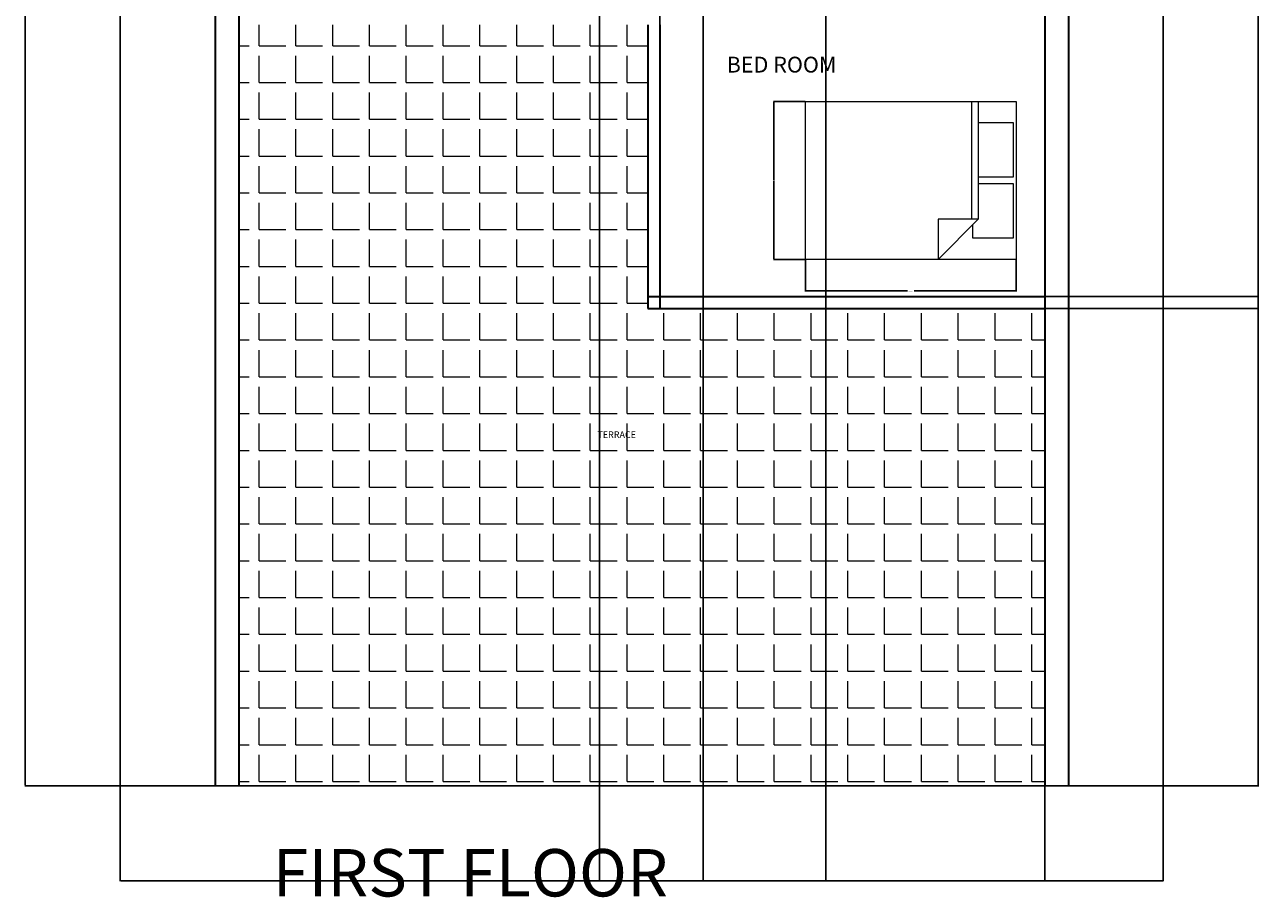
# Model space of a CAD drawing. Units: inches. Extents: x 2621 to 3621, y 1701 to 2465.
# Tile 5 of 6: x 3152 to 3621, y 1702 to 2034. Entities that reach past the tile are written whole.
import ezdxf

# ---------------------------------------------------------------- set-up
doc = ezdxf.new("R2010")
doc.units = ezdxf.units.IN
for name, color, linetype, lineweight in [('A-ANNO-DIMS', 2, 'Continuous', 18), ('A-ANNO-TEXT', 7, 'Continuous', 25), ('A-AREA-IDEN', 7, 'Continuous', 18), ('A-FLOR-PATT', 252, 'Continuous', 13), ('A-FURN', 8, 'Continuous', 18), ('A-WALL', 7, 'Continuous', 35), ('C-PROP', 8, 'Continuous', 25)]:
    doc.layers.add(name, color=color, linetype=linetype, lineweight=lineweight)
doc.styles.get("Standard").update_dxf_attribs({"font": 'arial.ttf'})
doc.dimstyles.get("Standard").update_dxf_attribs({"dimtxt": 0.18, "dimasz": 0.18, "dimexe": 0.18, "dimexo": 0.0625, "dimgap": 0.09, "dimtad": 0, "dimtih": 1, "dimtoh": 1, "dimdec": 4, "dimzin": 0, "dimdsep": 46, "dimtxsty": 'Standard', "dimcen": 0.09, "dimadec": 0, "dimazin": 0, "dimtfac": 1, "dimtdec": 4, "dimtofl": 0, "dimtmove": 0, "dimatfit": 3, "dimfxl": 1, "dimtolj": 1, "dimtzin": 0, "dimarcsym": 0})

# ---------------------------------------------------------------- blocks, each defined once
blk = doc.blocks.new('Bed - Queen')
for p, q in [((0, -80.00003), (0, 0)), ((0, 0), (59.99999, 0)), ((59.99999, 0), (59.99999, -80.00003)), ((7.99999, -1.2), (28.79998, -1.2)), ((7.99999, -14.4), (7.99999, -1.2)), ((28.79998, -1.2), (28.79998, -14.4)), ((31.19999, -1.2), (51.99999, -1.2)), ((31.19999, -14.4), (31.19999, -1.2)), ((51.99999, -1.2), (51.99999, -16.4)), ((0, -14.4), (44.8, -14.4)), ((44.8, -16.8), (0, -16.8)), ((59.99999, -29.6), (44.8, -14.4)), ((44.8, -14.4), (44.8, -29.6)), ((51.99999, -16.4), (46.79936, -16.4)), ((44.8, -29.6), (59.99999, -29.6)), ((59.99999, -80.00003), (0, -80.00003))]:
    blk.add_line(p, q)
blk = doc.blocks.new('LOT-33X57')
for p, q in [((0, 684), (396, 684)), ((0, 0), (0, 684)), ((396, 684), (396, 0)), ((396, 0), (0, 0))]:
    blk.add_line(p, q)
blk = doc.blocks.new('*D15')
at = {"layer": 'A-ANNO-DIMS', "color": 0, "lineweight": -2, "transparency": 16777216}
for p, q in [((3448.49, 1944.46), (3448.49, 1932.34)), ((3528.49, 1944.46), (3528.49, 1932.34)), ((3448.67, 1932.52), (3487.18, 1932.52)), ((3528.31, 1932.52), (3489.79, 1932.52))]:
    blk.add_line(p, q, dxfattribs=at)
at = {"layer": 'A-ANNO-DIMS', "color": 0, "transparency": 16777216}
for points in [[(3448.67, 1932.55), (3448.67, 1932.49), (3448.49, 1932.52)], [(3528.31, 1932.55), (3528.31, 1932.49), (3528.49, 1932.52)]]:
    blk.add_solid(points, dxfattribs=at)
at = {"layer": 'Defpoints', "color": 0, "transparency": 16777216}
for p in [(3448.49, 1944.52), (3528.49, 1944.52), (3528.49, 1932.52)]:
    blk.add_point(p, dxfattribs=at)
at = {"layer": 'A-ANNO-DIMS', "color": 0, "transparency": 16777216, "insert": (3488.49, 1932.52), "char_height": 0.18, "attachment_point": 5}
blk.add_mtext('\\A1;QUEEN BED 80 TYP.', dxfattribs=at)
blk = doc.blocks.new('*D16')
at = {"layer": 'A-ANNO-DIMS', "color": 0, "lineweight": -2, "transparency": 16777216}
for p, q in [((3448.43, 2004.52), (3436.31, 2004.52)), ((3436.49, 2004.34), (3436.49, 1974.7)), ((3436.49, 1944.7), (3436.49, 1974.34)), ((3448.43, 1944.52), (3436.31, 1944.52))]:
    blk.add_line(p, q, dxfattribs=at)
at = {"layer": 'A-ANNO-DIMS', "color": 0, "transparency": 16777216}
for points in [[(3436.46, 2004.34), (3436.52, 2004.34), (3436.49, 2004.52)], [(3436.46, 1944.7), (3436.52, 1944.7), (3436.49, 1944.52)]]:
    blk.add_solid(points, dxfattribs=at)
at = {"layer": 'Defpoints', "color": 0, "transparency": 16777216}
for p in [(3448.49, 2004.52), (3436.49, 1944.52), (3448.49, 1944.52)]:
    blk.add_point(p, dxfattribs=at)
at = {"layer": 'A-ANNO-DIMS', "color": 0, "transparency": 16777216, "insert": (3436.49, 1974.52), "char_height": 0.18, "attachment_point": 5}
blk.add_mtext('\\A1;60 TYP.', dxfattribs=at)
blk = doc.blocks.new('*D63')
at = {"layer": 'A-ANNO-DIMS', "color": 0, "lineweight": -2, "transparency": 16777216}
for p, q in [((3188.33, 1744.56), (3188.33, 1708.36)), ((3584.33, 1744.56), (3584.33, 1708.36)), ((3188.51, 1708.54), (3386.05, 1708.54)), ((3584.15, 1708.54), (3386.62, 1708.54))]:
    blk.add_line(p, q, dxfattribs=at)
at = {"layer": 'A-ANNO-DIMS', "color": 0, "transparency": 16777216}
for points in [[(3188.51, 1708.57), (3188.51, 1708.51), (3188.33, 1708.54)], [(3584.15, 1708.57), (3584.15, 1708.51), (3584.33, 1708.54)]]:
    blk.add_solid(points, dxfattribs=at)
at = {"layer": 'Defpoints', "color": 0, "transparency": 16777216}
for p in [(3188.33, 1744.63), (3584.33, 1744.63), (3584.33, 1708.54)]:
    blk.add_point(p, dxfattribs=at)
at = {"layer": 'A-ANNO-DIMS', "color": 0, "transparency": 16777216, "insert": (3386.33, 1708.54), "char_height": 0.18, "attachment_point": 5}
blk.add_mtext('\\A1;396', dxfattribs=at)
blk = doc.blocks.new('*D64')
at = {"layer": 'A-ANNO-DIMS', "color": 0, "lineweight": -2, "transparency": 16777216}
for p, q in [((3188.27, 2428.63), (3152.07, 2428.63)), ((3152.25, 2428.45), (3152.25, 2086.81)), ((3152.25, 1744.81), (3152.25, 2086.44)), ((3188.27, 1744.63), (3152.07, 1744.63))]:
    blk.add_line(p, q, dxfattribs=at)
at = {"layer": 'A-ANNO-DIMS', "color": 0, "transparency": 16777216}
for points in [[(3152.22, 2428.45), (3152.28, 2428.45), (3152.25, 2428.63)], [(3152.22, 1744.81), (3152.28, 1744.81), (3152.25, 1744.63)]]:
    blk.add_solid(points, dxfattribs=at)
at = {"layer": 'Defpoints', "color": 0, "transparency": 16777216}
for p in [(3152.25, 2428.63), (3188.33, 2428.63), (3188.33, 1744.63)]:
    blk.add_point(p, dxfattribs=at)
at = {"layer": 'A-ANNO-DIMS', "color": 0, "transparency": 16777216, "insert": (3152.25, 2086.63), "char_height": 0.18, "attachment_point": 5}
blk.add_mtext('\\A1;684', dxfattribs=at)
blk = doc.blocks.new('*D66')
at = {"layer": 'A-ANNO-DIMS', "color": 0, "lineweight": -2, "transparency": 16777216}
for p, q in [((3548.4, 2392.63), (3620.6, 2392.63)), ((3620.42, 2392.45), (3620.42, 2068.81)), ((3620.42, 1744.81), (3620.42, 2068.44)), ((3548.4, 1744.63), (3620.6, 1744.63))]:
    blk.add_line(p, q, dxfattribs=at)
at = {"layer": 'A-ANNO-DIMS', "color": 0, "transparency": 16777216}
for points in [[(3620.39, 2392.45), (3620.45, 2392.45), (3620.42, 2392.63)], [(3620.39, 1744.81), (3620.45, 1744.81), (3620.42, 1744.63)]]:
    blk.add_solid(points, dxfattribs=at)
at = {"layer": 'Defpoints', "color": 0, "transparency": 16777216}
for p in [(3548.33, 2392.63), (3620.42, 2392.63), (3548.33, 1744.63)]:
    blk.add_point(p, dxfattribs=at)
at = {"layer": 'A-ANNO-DIMS', "color": 0, "transparency": 16777216, "insert": (3620.42, 2068.63), "char_height": 0.18, "attachment_point": 5}
blk.add_mtext('\\A1;648', dxfattribs=at)
blk = doc.blocks.new('*D68')
at = {"layer": 'A-ANNO-DIMS', "color": 0, "lineweight": -2, "transparency": 16777216}
for p, q in [((3370.34, 2383.56), (3370.34, 1708.36)), ((3409.59, 2383.56), (3409.59, 1708.36)), ((3370.52, 1708.54), (3389.57, 1708.54)), ((3409.41, 1708.54), (3390.36, 1708.54))]:
    blk.add_line(p, q, dxfattribs=at)
at = {"layer": 'A-ANNO-DIMS', "color": 0, "transparency": 16777216}
for points in [[(3370.52, 1708.57), (3370.52, 1708.51), (3370.34, 1708.54)], [(3409.41, 1708.57), (3409.41, 1708.51), (3409.59, 1708.54)]]:
    blk.add_solid(points, dxfattribs=at)
at = {"layer": 'Defpoints', "color": 0, "transparency": 16777216}
for p in [(3370.34, 2383.63), (3409.59, 2383.63), (3409.59, 1708.54)]:
    blk.add_point(p, dxfattribs=at)
at = {"layer": 'A-ANNO-DIMS', "color": 0, "transparency": 16777216, "insert": (3389.97, 1708.54), "char_height": 0.18, "attachment_point": 5}
blk.add_mtext('\\A1;39.25', dxfattribs=at)
blk = doc.blocks.new('*D76')
at = {"layer": 'A-ANNO-DIMS', "color": 0, "lineweight": -2, "transparency": 16777216}
for p, q in [((3456.23, 2062.74), (3456.23, 1708.36)), ((3539.33, 2062.74), (3539.33, 1708.36)), ((3456.41, 1708.54), (3497.47, 1708.54)), ((3539.15, 1708.54), (3498.09, 1708.54))]:
    blk.add_line(p, q, dxfattribs=at)
at = {"layer": 'A-ANNO-DIMS', "color": 0, "transparency": 16777216}
for points in [[(3456.41, 1708.57), (3456.41, 1708.51), (3456.23, 1708.54)], [(3539.15, 1708.57), (3539.15, 1708.51), (3539.33, 1708.54)]]:
    blk.add_solid(points, dxfattribs=at)
at = {"layer": 'Defpoints', "color": 0, "transparency": 16777216}
for p in [(3456.23, 2062.8), (3539.33, 2062.8), (3539.33, 1708.54)]:
    blk.add_point(p, dxfattribs=at)
at = {"layer": 'A-ANNO-DIMS', "color": 0, "transparency": 16777216, "insert": (3497.78, 1708.54), "char_height": 0.18, "attachment_point": 5}
blk.add_mtext('\\A1;83.1', dxfattribs=at)
blk = doc.blocks.new('*D78')
at = {"layer": 'A-ANNO-DIMS', "color": 0, "lineweight": -2, "transparency": 16777216}
for p, q in [((3393.19, 1925.94), (3393.19, 2464.89)), ((3393.37, 2464.71), (3465.81, 2464.71)), ((3539.15, 2464.71), (3466.72, 2464.71)), ((3539.33, 1930.44), (3539.33, 2464.89))]:
    blk.add_line(p, q, dxfattribs=at)
at = {"layer": 'A-ANNO-DIMS', "color": 0, "transparency": 16777216}
for points in [[(3393.37, 2464.74), (3393.37, 2464.68), (3393.19, 2464.71)], [(3539.15, 2464.74), (3539.15, 2464.68), (3539.33, 2464.71)]]:
    blk.add_solid(points, dxfattribs=at)
at = {"layer": 'Defpoints', "color": 0, "transparency": 16777216}
for p in [(3539.33, 2464.71), (3539.33, 1930.38), (3393.19, 1925.88)]:
    blk.add_point(p, dxfattribs=at)
at = {"layer": 'A-ANNO-DIMS', "color": 0, "transparency": 16777216, "insert": (3466.26, 2464.71), "char_height": 0.18, "attachment_point": 5}
blk.add_mtext('\\A1;146.14', dxfattribs=at)
blk = doc.blocks.new('*D79')
at = {"layer": 'A-ANNO-DIMS', "color": 0, "lineweight": -2, "transparency": 16777216}
for p, q in [((3539.4, 2062.8), (3620.6, 2062.8)), ((3620.42, 2062.62), (3620.42, 1996.77)), ((3620.42, 1930.56), (3620.42, 1996.41)), ((3539.4, 1930.38), (3620.6, 1930.38))]:
    blk.add_line(p, q, dxfattribs=at)
at = {"layer": 'A-ANNO-DIMS', "color": 0, "transparency": 16777216}
for points in [[(3620.39, 2062.62), (3620.45, 2062.62), (3620.42, 2062.8)], [(3620.39, 1930.56), (3620.45, 1930.56), (3620.42, 1930.38)]]:
    blk.add_solid(points, dxfattribs=at)
at = {"layer": 'Defpoints', "color": 0, "transparency": 16777216}
for p in [(3539.33, 2062.8), (3620.42, 2062.8), (3539.33, 1930.38)]:
    blk.add_point(p, dxfattribs=at)
at = {"layer": 'A-ANNO-DIMS', "color": 0, "transparency": 16777216, "insert": (3620.42, 1996.59), "char_height": 0.18, "attachment_point": 5}
blk.add_mtext('\\A1;132.42', dxfattribs=at)
blk = doc.blocks.new('*D80')
at = {"layer": 'A-ANNO-DIMS', "color": 0, "lineweight": -2, "transparency": 16777216}
for p, q in [((3539.4, 1925.88), (3620.6, 1925.88)), ((3620.42, 1925.7), (3620.42, 1835.44)), ((3620.42, 1744.81), (3620.42, 1835.07)), ((3539.4, 1744.63), (3620.6, 1744.63))]:
    blk.add_line(p, q, dxfattribs=at)
at = {"layer": 'A-ANNO-DIMS', "color": 0, "transparency": 16777216}
for points in [[(3620.39, 1925.7), (3620.45, 1925.7), (3620.42, 1925.88)], [(3620.39, 1744.81), (3620.45, 1744.81), (3620.42, 1744.63)]]:
    blk.add_solid(points, dxfattribs=at)
at = {"layer": 'Defpoints', "color": 0, "transparency": 16777216}
for p in [(3539.33, 1925.88), (3620.42, 1925.88), (3539.33, 1744.63)]:
    blk.add_point(p, dxfattribs=at)
at = {"layer": 'A-ANNO-DIMS', "color": 0, "transparency": 16777216, "insert": (3620.42, 1835.25), "char_height": 0.18, "attachment_point": 5}
blk.add_mtext('\\A1;181.26', dxfattribs=at)

msp = doc.modelspace()

# ---------------------------------------------------------------- hatches: boundary and pattern name
at = {"layer": 'A-FLOR-PATT'}
h = msp.add_hatch(dxfattribs=at)
h.set_pattern_fill('ANGLE', color=256, scale=2)
h.set_pattern_definition([(0, (0, 0), (0, 13.97), [10.16, -3.81]), (90, (0, 0), (-13.97, 9e-16), [10.16, -3.81])])
h.paths.add_polyline_path([(3233.335, 2383.626), (3233.335, 2215.626), (3366.0915, 2215.626), (3366.0915, 2383.626), (3344.3345, 2383.626), (3339.8345, 2383.626)])
h.paths.add_polyline_path([(3233.335, 2033.6278), (3233.335, 1895.6231), (3233.335, 1744.626), (3539.335, 1744.626), (3539.335, 1780.626), (3539.335, 1789.626), (3539.335, 1859.7646), (3539.335, 1862.3069), (3539.335, 1925.8819), (3388.6903, 1925.8819), (3388.6903, 2033.6278)])

# ---------------------------------------------------------------- linework, layer by layer
at = {"layer": 'A-WALL'}
for p, q in [((3224.335, 2428.626), (3224.335, 1891.1231)), ((3233.335, 2111.9772), (3233.335, 1895.6231)), ((3539.335, 2111.9772), (3539.335, 2015.622)), ((3548.335, 2111.9772), (3548.335, 1780.626)), ((3388.6903, 2033.6278), (3388.6903, 1925.8819)), ((3393.1903, 2033.6278), (3393.1903, 1925.8819)), ((3539.335, 2015.622), (3539.335, 2011.122)), ((3539.335, 2011.122), (3539.335, 1955.3016)), ((3539.335, 1955.3016), (3539.335, 1950.8016)), ((3539.335, 1950.8016), (3539.335, 1862.3069)), ((3388.6903, 1930.3819), (3539.335, 1930.3819)), ((3388.6903, 1925.8819), (3539.335, 1925.8819)), ((3233.335, 1895.6231), (3233.335, 1744.626)), ((3224.335, 1891.1231), (3224.335, 1744.626)), ((3539.335, 1862.3069), (3539.335, 1859.7646)), ((3539.335, 1859.7646), (3539.335, 1789.626)), ((3539.335, 1789.626), (3539.335, 1780.626)), ((3539.335, 1780.626), (3539.335, 1744.626)), ((3548.335, 1780.626), (3548.335, 1744.626))]:
    msp.add_line(p, q, dxfattribs=at)

# ---------------------------------------------------------------- block references
at = {"layer": 'A-FURN', "rotation": 270}
msp.add_blockref('Bed - Queen', (3528.4879, 2004.5213), dxfattribs=at)
at = {"layer": 'C-PROP'}
msp.add_blockref('LOT-33X57', (3188.3346, 1744.6265), dxfattribs=at)

# ---------------------------------------------------------------- texts
at = {"layer": 'A-ANNO-TEXT', "insert": (3246.1971, 1720.589), "char_height": 18, "attachment_point": 1}
msp.add_mtext_dynamic_manual_height_columns('FIRST FLOOR', width=483.442651, gutter_width=12.5, heights=[0], dxfattribs=at)
at = {"layer": 'A-AREA-IDEN', "attachment_point": 1}
for s, width, insert, char_height in [('BED ROOM', 49.051461, (3418.5714, 2021.4596), 6), ('TERRACE ', 54.244428, (3369.4942, 1879.2046), 2.5)]:
    msp.add_mtext_dynamic_manual_height_columns(s, width=width, gutter_width=12.5, heights=[0], dxfattribs=dict(at, insert=insert, char_height=char_height))

# ---------------------------------------------------------------- dimensions: what is measured, and where the dimension line sits
at = {"layer": 'A-ANNO-DIMS'}
for base, p1, p2, override, picture, middle in [((3539.335, 2464.708), (3393.1903, 1925.8819), (3539.335, 1930.3819), {"dimdec": 2, "dimlfac": 1, "dimrnd": 0, "dimzin": 0, "dimdsep": 46, "dimlunit": 2}, '*D78', (3466.2626, 2464.708)), ((3409.5915, 1708.544), (3370.3415, 2383.626), (3409.5915, 2383.626), {"dimdec": 2, "dimlfac": 1, "dimrnd": 0, "dimzin": 0, "dimdsep": 46, "dimlunit": 2}, '*D68', (3389.9665, 1708.544)), ((3539.335, 1708.544), (3456.2276, 2062.7992), (3539.335, 2062.7992), {"dimdec": 1, "dimlfac": 1, "dimrnd": 0, "dimzin": 0, "dimdsep": 46, "dimlunit": 2}, '*D76', (3497.7813, 1708.544)), ((3584.335, 1708.544), (3188.335, 1744.626), (3584.335, 1744.626), {"dimdec": 0, "dimlfac": 1, "dimrnd": 0, "dimzin": 0, "dimdsep": 46, "dimlunit": 2}, '*D63', (3386.335, 1708.544))]:
    dim = msp.add_linear_dim(base=base, p1=p1, p2=p2, dimstyle='Standard', override=override, dxfattribs=at)
    dim.commit()
    dim.dimension.update_dxf_attribs({"geometry": picture, "text_midpoint": middle})
for base, p1, p2, override, picture, middle in [((3152.253, 2428.626), (3188.335, 1744.626), (3188.335, 2428.626), {"dimdec": 0, "dimlfac": 1, "dimrnd": 0, "dimzin": 0, "dimdsep": 46, "dimlunit": 2}, '*D64', (3152.253, 2086.626)), ((3620.417, 2392.626), (3548.335, 1744.626), (3548.335, 2392.626), {"dimdec": 0, "dimlfac": 1, "dimrnd": 0, "dimzin": 0, "dimdsep": 46, "dimlunit": 2}, '*D66', (3620.417, 2068.626)), ((3620.417, 2062.7992), (3539.335, 1930.3819), (3539.335, 2062.7992), {"dimdec": 2, "dimlfac": 1, "dimrnd": 0, "dimzin": 0, "dimdsep": 46, "dimlunit": 2}, '*D79', (3620.417, 1996.5905)), ((3620.417, 1925.8819), (3539.335, 1744.626), (3539.335, 1925.8819), {"dimdec": 2, "dimlfac": 1, "dimrnd": 0, "dimzin": 0, "dimdsep": 46, "dimlunit": 2}, '*D80', (3620.417, 1835.2539))]:
    dim = msp.add_linear_dim(base=base, p1=p1, p2=p2, angle=90, dimstyle='Standard', override=override, dxfattribs=at)
    dim.commit()
    dim.dimension.update_dxf_attribs({"geometry": picture, "text_midpoint": middle})
dim = msp.add_linear_dim(base=(3436.4879, 1944.5213), p1=(3448.4879, 2004.5213), p2=(3448.4879, 1944.5213), angle=270, text='<> TYP.', dimstyle='Standard', override={"dimdec": 0, "dimlfac": 1, "dimrnd": 0, "dimzin": 0, "dimdsep": 46, "dimlunit": 2}, dxfattribs=at)
dim.commit()
dim.dimension.update_dxf_attribs({"geometry": '*D16', "text_midpoint": (3436.4879, 1974.5213)})
dim = msp.add_linear_dim(base=(3528.4879, 1932.5213), p1=(3448.4879, 1944.5213), p2=(3528.4879, 1944.5213), text='QUEEN BED <> TYP.', dimstyle='Standard', override={"dimdec": 0, "dimlfac": 1, "dimrnd": 0, "dimzin": 0, "dimdsep": 46, "dimlunit": 2}, dxfattribs=at)
dim.commit()
dim.dimension.update_dxf_attribs({"geometry": '*D15', "text_midpoint": (3488.4879, 1932.5213)})

doc.saveas('drawing.dxf')
